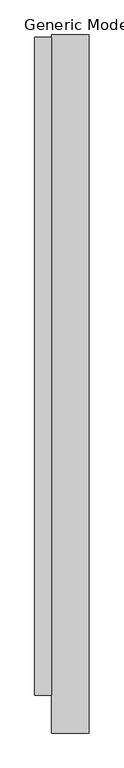
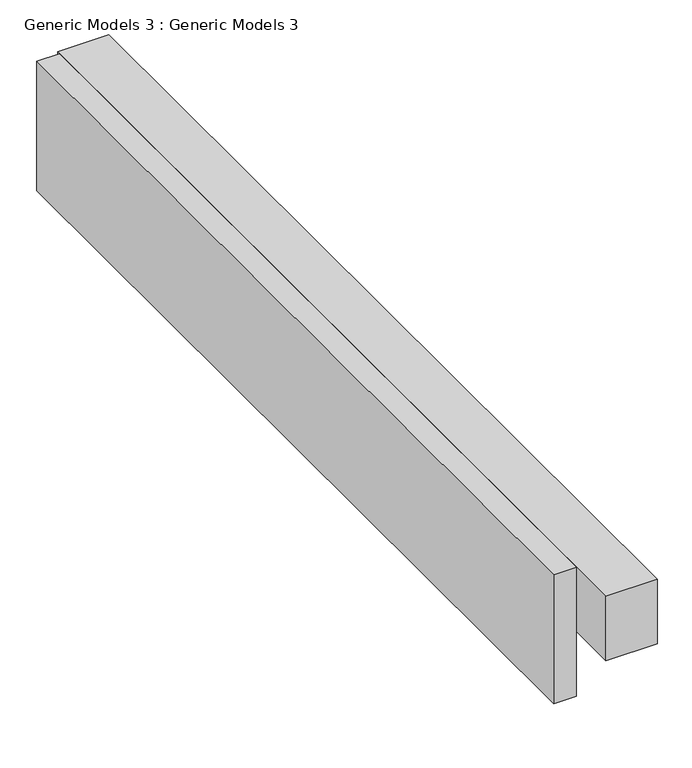
"""IFC4 building model written with IfcOpenShell, lengths in millimetres: proxy geometry, Generic Models 3 : Generic Models 3."""

from ifc_helpers import new_model, si_unit, frame, origin, place, context, project, spatial, polyline, outline, extrude, source, transform, mapped, element, save


def generic_models_3_generic_models_3_e8135b9d(model_context):
    return source(origin(), model_context, "Body", "SweptSolid", [
        extrude(outline(polyline([(-7274.9953834, 4735.8552287), (-7173.3953834, 4735.8552287), (-7173.3953834, 740.1262137), (-7274.9953834, 740.1262137), (-7274.9953834, 4735.8552287)])), frame((0.0, 0.0, 5638.8), z_axis=(0.0, 0.0, 1.0), x_axis=(1.0, 0.0, 0.0)), (0.0, 0.0, 1.0), 609.6),
        extrude(outline(polyline([(-6944.7953834, 4751.3245311), (-6944.7953834, 511.5262137), (-7173.3953834, 511.5262137), (-7173.3953834, 4751.3245311), (-6944.7953834, 4751.3245311)])), frame((0.0, 0.0, 5945.6852238), z_axis=(0.0, 0.0, 1.0), x_axis=(1.0, 0.0, 0.0)), (0.0, 0.0, 1.0), 302.7147762),
    ])


if __name__ == "__main__":
    model = new_model("IFC4")
    model_context = context("Model", 3, world=origin())
    ifc_project = project(units=[si_unit("LENGTHUNIT", "METRE", prefix="MILLI")], contexts=[model_context])
    site = spatial("IfcSite", under=ifc_project)
    building = spatial("IfcBuilding", under=site)
    placement = place(None, origin())
    generic_models_3_generic_models_3_shape = generic_models_3_generic_models_3_e8135b9d(model_context)
    element("IfcBuildingElementProxy", 1, Name="Generic Models 3 : Generic Models 3", ObjectType="Generic Models 3 : Generic Models 3", at=placement, inside=building, context=model_context, shape_type="MappedRepresentation", body=[
        mapped(generic_models_3_generic_models_3_shape, transform((0.0, 0.0, 0.0), x_axis=(1.0, 0.0, 0.0), y_axis=(0.0, 1.0, 0.0), z_axis=(0.0, 0.0, 1.0))),
    ])
    save(model, "model.ifc")

# Revit data of these elements
# Element 1 (IfcBuildingElementProxy, "Generic Models 3 : Generic Models 3")
#   Materials on its faces: "Asphalt, Pavement, Light Grey"
# Materials
#   "Asphalt, Pavement, Light Grey": class "Generic", colour RGB 120 120 120, transparency 0, Description = "Asphalt or tarmac paving", Cost = 0
